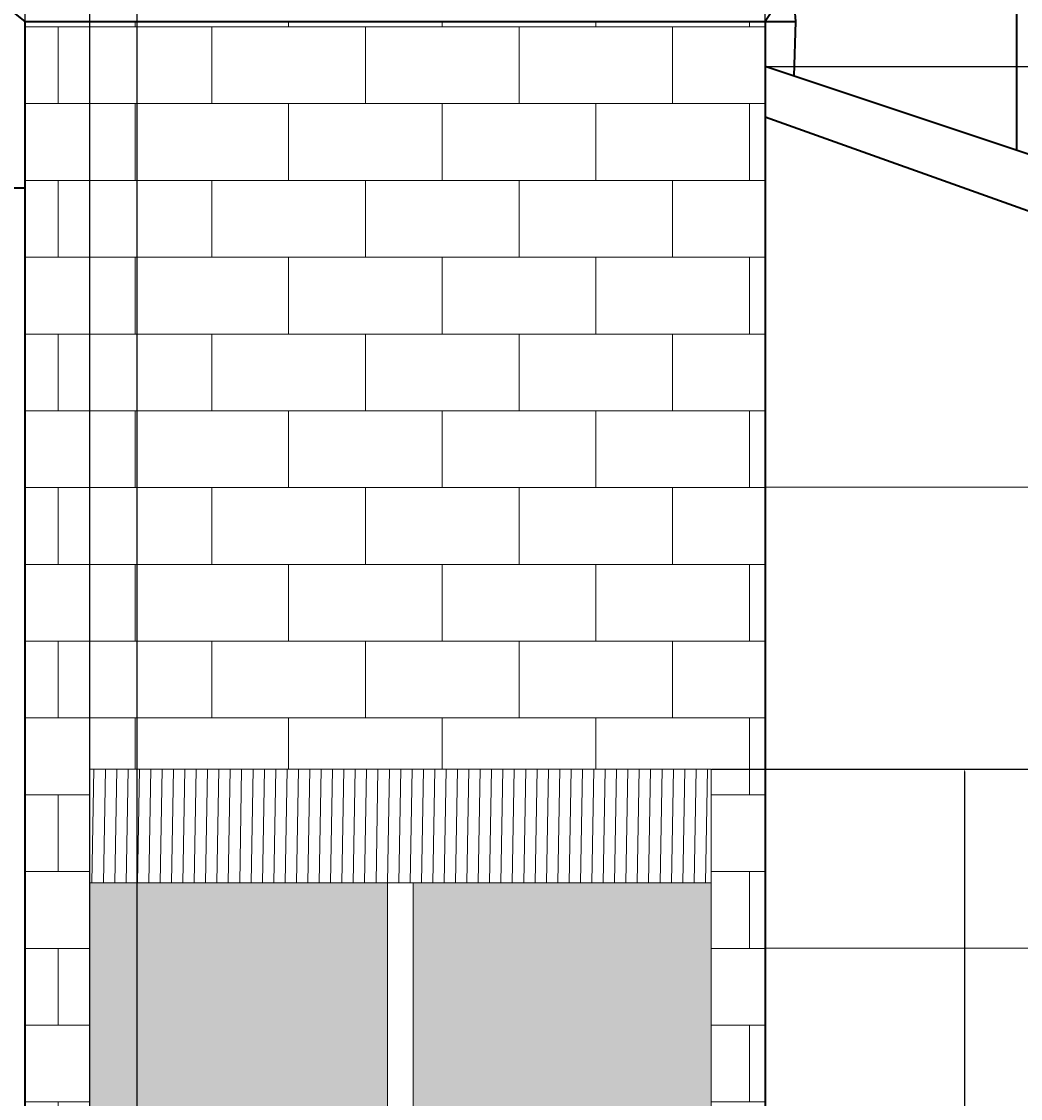
# Model space of a CAD drawing. Units: inches. Extents: x -26 to 776, y -22 to 650.
# Tile 34 of 62: x 231 to 309, y 420 to 504. Entities that reach past the tile are written whole.
import ezdxf

# ---------------------------------------------------------------- set-up
doc = ezdxf.new("R2010")
doc.units = ezdxf.units.IN
doc.header["$MEASUREMENT"] = 0
for name, color, linetype, lineweight in [('A-ANNO-DIMS', 2, 'Continuous', 18), ('A-DETL-PATT', 8, 'Continuous', 13), ('A-GLAZ', 4, 'Continuous', 18), ('A-GLAZ-PATT', 9, 'Continuous', 13), ('A-ROOF', 7, 'Continuous', 35), ('A-WALL', 7, 'Continuous', 35), ('A-WALL-PATT', 8, 'Continuous', 13)]:
    doc.layers.add(name, color=color, linetype=linetype, lineweight=lineweight)
doc.styles.get("Standard").update_dxf_attribs({"font": 'arial.ttf'})
doc.dimstyles.get("Standard").update_dxf_attribs({"dimtxt": 0.5625, "dimasz": 0.18, "dimexe": 0.18, "dimexo": 0.0625, "dimgap": 0.09, "dimtad": 0, "dimtih": 1, "dimtoh": 1, "dimdec": 4, "dimzin": 0, "dimdsep": 46, "dimlunit": 4, "dimtxsty": 'Standard', "dimcen": 0.09, "dimadec": 0, "dimazin": 0, "dimtfac": 1, "dimtdec": 4, "dimtofl": 0, "dimtmove": 0, "dimatfit": 3, "dimfxl": 1, "dimtolj": 1, "dimtzin": 0, "dimarcsym": 0})

# ---------------------------------------------------------------- blocks, each defined once
blk = doc.blocks.new('WIN-ELEV-2X4-HEAD')
for p, q in [((0, 123), (0, 131.888)), ((0, 131.888), (48.553, 131.888)), ((48.553, 131.888), (48.553, 123)), ((23.276, 0), (23.276, 123)), ((25.276, 0), (25.276, 123))]:
    blk.add_line(p, q)
blk.add_lwpolyline([(48.553, 0), (0, 0), (0, 123), (48.553, 123)], close=True)
blk = doc.blocks.new('*D9')
at = {"layer": 'A-ANNO-DIMS', "color": 0, "lineweight": -2, "transparency": 16777216}
for p, q in [((285.08, 446.006), (304.981, 446.006)), ((304.801, 445.826), (304.801, 380.444)), ((304.801, 314.299), (304.801, 379.681)), ((285.08, 314.119), (304.981, 314.119))]:
    blk.add_line(p, q, dxfattribs=at)
at = {"layer": 'A-ANNO-DIMS', "color": 0, "transparency": 16777216}
for points in [[(304.771, 445.826), (304.831, 445.826), (304.801, 446.006)], [(304.771, 314.299), (304.831, 314.299), (304.801, 314.119)]]:
    blk.add_solid(points, dxfattribs=at)
at = {"layer": 'Defpoints', "color": 0, "transparency": 16777216}
for p in [(285.018, 446.006), (304.801, 446.006), (285.018, 314.119)]:
    blk.add_point(p, dxfattribs=at)
at = {"layer": 'A-ANNO-DIMS', "color": 0, "transparency": 16777216, "insert": (304.801, 380.063), "char_height": 0.5625, "attachment_point": 5}
blk.add_mtext('\\A1;NARROW WINDOW 132 TYP.', dxfattribs=at)
blk = doc.blocks.new('*D15')
at = {"layer": 'A-ANNO-DIMS', "color": 0, "lineweight": -2, "transparency": 16777216}
for p, q in [((11.107, 491.489), (11.107, 649.856)), ((11.287, 649.676), (120.222, 649.676)), ((231.245, 649.676), (122.31, 649.676)), ((231.425, 491.489), (231.425, 649.856))]:
    blk.add_line(p, q, dxfattribs=at)
at = {"layer": 'A-ANNO-DIMS', "color": 0, "transparency": 16777216}
for points in [[(11.287, 649.706), (11.287, 649.646), (11.107, 649.676)], [(231.245, 649.706), (231.245, 649.646), (231.425, 649.676)]]:
    blk.add_solid(points, dxfattribs=at)
at = {"layer": 'Defpoints', "color": 0, "transparency": 16777216}
for p in [(231.425, 649.676), (11.107, 491.427), (231.425, 491.427)]:
    blk.add_point(p, dxfattribs=at)
at = {"layer": 'A-ANNO-DIMS', "color": 0, "transparency": 16777216, "insert": (121.266, 649.676), "char_height": 0.5625, "attachment_point": 5}
blk.add_mtext('\\A1;220.3', dxfattribs=at)
blk = doc.blocks.new('*D31')
at = {"layer": 'A-ANNO-DIMS', "color": 0, "lineweight": -2, "transparency": 16777216}
for p, q in [((289.305, 500.896), (775.335, 500.896)), ((775.155, 500.716), (775.155, 473.828)), ((775.155, 446.186), (775.155, 473.074)), ((285.08, 446.006), (775.335, 446.006))]:
    blk.add_line(p, q, dxfattribs=at)
at = {"layer": 'A-ANNO-DIMS', "color": 0, "transparency": 16777216}
for points in [[(775.125, 500.716), (775.185, 500.716), (775.155, 500.896)], [(775.125, 446.186), (775.185, 446.186), (775.155, 446.006)]]:
    blk.add_solid(points, dxfattribs=at)
at = {"layer": 'Defpoints', "color": 0, "transparency": 16777216}
for p in [(289.242, 500.896), (775.155, 500.896), (285.018, 446.006)]:
    blk.add_point(p, dxfattribs=at)
at = {"layer": 'A-ANNO-DIMS', "color": 0, "transparency": 16777216, "insert": (775.155, 473.451), "char_height": 0.5625, "attachment_point": 5}
blk.add_mtext('\\A1;54.89', dxfattribs=at)
blk = doc.blocks.new('*D34')
at = {"layer": 'A-ANNO-DIMS', "color": 0, "lineweight": -2, "transparency": 16777216}
for p, q in [((228.573, 528.296), (228.573, -21.315)), ((357.303, 528.361), (357.303, -21.315)), ((228.753, -21.135), (291.707, -21.135)), ((357.123, -21.135), (294.17, -21.135))]:
    blk.add_line(p, q, dxfattribs=at)
at = {"layer": 'A-ANNO-DIMS', "color": 0, "transparency": 16777216}
for points in [[(228.753, -21.105), (228.753, -21.165), (228.573, -21.135)], [(357.123, -21.105), (357.123, -21.165), (357.303, -21.135)]]:
    blk.add_solid(points, dxfattribs=at)
at = {"layer": 'Defpoints', "color": 0, "transparency": 16777216}
for p in [(357.303, 528.423), (228.573, 528.358), (357.303, -21.135)]:
    blk.add_point(p, dxfattribs=at)
at = {"layer": 'A-ANNO-DIMS', "color": 0, "transparency": 16777216, "insert": (292.938, -21.135), "char_height": 0.5625, "attachment_point": 5}
blk.add_mtext('\\A1;128.73', dxfattribs=at)
blk = doc.blocks.new('*D39')
at = {"layer": 'A-ANNO-DIMS', "color": 0, "lineweight": -2, "transparency": 16777216}
for p, q in [((289.242, 15.545), (289.242, 649.856)), ((289.422, 649.676), (356.478, 649.676)), ((425.563, 649.676), (358.508, 649.676)), ((425.743, 15.545), (425.743, 649.856))]:
    blk.add_line(p, q, dxfattribs=at)
at = {"layer": 'A-ANNO-DIMS', "color": 0, "transparency": 16777216}
for points in [[(289.422, 649.706), (289.422, 649.646), (289.242, 649.676)], [(425.563, 649.706), (425.563, 649.646), (425.743, 649.676)]]:
    blk.add_solid(points, dxfattribs=at)
at = {"layer": 'Defpoints', "color": 0, "transparency": 16777216}
for p in [(425.743, 649.676), (289.242, 15.482), (425.743, 15.482)]:
    blk.add_point(p, dxfattribs=at)
at = {"layer": 'A-ANNO-DIMS', "color": 0, "transparency": 16777216, "insert": (357.493, 649.676), "char_height": 0.5625, "attachment_point": 5}
blk.add_mtext('\\A1;136.5', dxfattribs=at)
blk = doc.blocks.new('*D43')
at = {"layer": 'A-ANNO-DIMS', "color": 0, "lineweight": -2, "transparency": 16777216}
for p, q in [((231.425, 159.545), (231.425, 649.856)), ((231.605, 649.676), (233.125, 649.676)), ((236.285, 649.676), (234.764, 649.676)), ((236.465, 171.48), (236.465, 649.856))]:
    blk.add_line(p, q, dxfattribs=at)
at = {"layer": 'A-ANNO-DIMS', "color": 0, "transparency": 16777216}
for points in [[(231.605, 649.706), (231.605, 649.646), (231.425, 649.676)], [(236.285, 649.706), (236.285, 649.646), (236.465, 649.676)]]:
    blk.add_solid(points, dxfattribs=at)
at = {"layer": 'Defpoints', "color": 0, "transparency": 16777216}
for p in [(236.465, 649.676), (236.465, 171.417), (231.425, 159.482)]:
    blk.add_point(p, dxfattribs=at)
at = {"layer": 'A-ANNO-DIMS', "color": 0, "transparency": 16777216, "insert": (233.945, 649.676), "char_height": 0.5625, "attachment_point": 5}
blk.add_mtext('\\A1;5.04', dxfattribs=at)
blk = doc.blocks.new('*D44')
at = {"layer": 'A-ANNO-DIMS', "color": 0, "lineweight": -2, "transparency": 16777216}
for p, q in [((231.425, 15.545), (231.425, 649.856)), ((231.605, 649.676), (234.975, 649.676)), ((239.985, 649.676), (236.615, 649.676)), ((240.165, 26.486), (240.165, 649.856))]:
    blk.add_line(p, q, dxfattribs=at)
at = {"layer": 'A-ANNO-DIMS', "color": 0, "transparency": 16777216}
for points in [[(231.605, 649.706), (231.605, 649.646), (231.425, 649.676)], [(239.985, 649.706), (239.985, 649.646), (240.165, 649.676)]]:
    blk.add_solid(points, dxfattribs=at)
at = {"layer": 'Defpoints', "color": 0, "transparency": 16777216}
for p in [(240.165, 649.676), (240.165, 26.424), (231.425, 15.482)]:
    blk.add_point(p, dxfattribs=at)
at = {"layer": 'A-ANNO-DIMS', "color": 0, "transparency": 16777216, "insert": (235.795, 649.676), "char_height": 0.5625, "attachment_point": 5}
blk.add_mtext('\\A1;8.74', dxfattribs=at)

msp = doc.modelspace()

# ---------------------------------------------------------------- hatches: boundary and pattern name
at = {"layer": 'A-DETL-PATT'}
h = msp.add_hatch(dxfattribs=at)
h.set_pattern_fill('ANSI31', color=256, scale=7.1, angle=44)
h.paths.add_polyline_path([(231.4249, 197.3298), (216.1056, 197.3298), (216.1056, 159.4824), (231.4249, 159.4824)])
h.paths.add_polyline_path([(236.4647, 197.3298), (231.4249, 197.3298), (231.4249, 159.4824), (276.1134, 159.4824), (276.1134, 171.4173), (236.4647, 171.4173)])
h.paths.add_polyline_path([(259.7413, 197.3298), (236.4647, 197.3298), (236.4647, 171.4173), (259.7413, 171.4173)], flags=17)
h.paths.add_polyline_path([(276.1134, 197.3298), (261.7413, 197.3298), (261.7413, 171.4173), (276.1134, 171.4173)], flags=17)
h.paths.add_polyline_path([(217.9529, 147.0781), (22.8891, 147.0781), (22.8891, 138.3844), (217.9529, 138.3844)])
h.paths.add_polyline_path([(285.0179, 152.3087), (285.0179, 159.4824), (231.4249, 159.4824), (240.1654, 144.8359), (280.6173, 144.8359)])
h.paths.add_polyline_path([(280.6173, 144.8359), (240.1654, 144.8359), (240.1654, 26.4239), (280.6173, 26.4239)])
h.paths.add_polyline_path([(274.6644, 134.8811), (274.6644, 34.0885), (245.7207, 34.0885), (245.7207, 134.8811)], flags=16)
h.paths.add_polyline_path([(285.0179, 303.3046), (236.4647, 303.3046), (236.4647, 294.4171), (285.0179, 294.4171)])
h.paths.add_polyline_path([(285.0179, 446.0063), (236.4647, 446.0063), (236.4647, 437.1188), (285.0179, 437.1188)])
at = {"layer": 'A-GLAZ-PATT'}
h = msp.add_hatch(dxfattribs=at)
h.set_pattern_fill('GOST_GLASS', color=256, scale=0.75)
h.set_pattern_definition([(45, (0, 0), (6.36396, 0), [3.75, -5.25]), (45, (1.591, 0), (6.36396, 0), [1.5, -7.5]), (45, (0, 1.591), (6.36396, 0), [1.5, -7.5])])
h.paths.add_polyline_path([(115.8402, 198.8773), (93.6448, 198.8773), (93.6448, 173.9734), (115.8402, 173.9734)])
h.paths.add_polyline_path([(144.1571, 198.8773), (115.8402, 198.8773), (115.8402, 173.9734), (144.1571, 173.9734)])
h.paths.add_polyline_path([(115.8402, 224.3396), (93.6448, 224.3396), (93.6448, 198.8773), (115.8402, 198.8773)])
h.paths.add_polyline_path([(144.1571, 248.4417), (115.8402, 248.4417), (115.8402, 224.3396), (144.1571, 224.3396)])
h.paths.add_polyline_path([(144.1571, 224.3396), (115.8402, 224.3396), (115.8402, 198.8773), (144.1571, 198.8773)])
h.paths.add_polyline_path([(170.5449, 224.3396), (144.1571, 224.3396), (144.1571, 198.8773), (170.5449, 198.8773)])
h.paths.add_polyline_path([(170.5449, 198.8773), (144.1571, 198.8773), (144.1571, 173.9734), (170.5449, 173.9734)])
h.paths.add_polyline_path([(194.6694, 198.8773), (170.5449, 198.8773), (170.5449, 173.9734), (194.6694, 173.9734)])
h.paths.add_polyline_path([(194.6694, 224.3396), (170.5449, 224.3396), (170.5449, 198.8773), (194.6694, 198.8773)])
h.paths.add_polyline_path([(194.6694, 248.4417), (170.5449, 248.4417), (170.5449, 224.3396), (194.6694, 224.3396)])
h.paths.add_polyline_path([(170.5449, 248.4417), (144.1571, 248.4417), (144.1571, 224.3396), (170.5449, 224.3396)])
h.paths.add_polyline_path([(144.1571, 269.3091), (115.8402, 269.3091), (115.8402, 248.4417), (144.1571, 248.4417)])
h.paths.add_polyline_path([(115.8402, 269.3091), (93.6448, 269.3091), (93.6448, 248.4417), (115.8402, 248.4417)])
h.paths.add_polyline_path([(115.8402, 248.4417), (93.6448, 248.4417), (93.6448, 224.3396), (115.8402, 224.3396)])
h.paths.add_polyline_path([(170.5449, 269.3091), (144.1571, 269.3091), (144.1571, 248.4417), (170.5449, 248.4417)])
h.paths.add_polyline_path([(194.6694, 269.3091), (170.5449, 269.3091), (170.5449, 248.4417), (194.6694, 248.4417)])
h.paths.add_polyline_path([(259.7413, 294.4171), (236.4647, 294.4171), (236.4647, 266.1888), (259.7413, 266.1888)])
h.paths.add_polyline_path([(285.0179, 294.4171), (261.7413, 294.4171), (261.7413, 266.1888), (285.0179, 266.1888)])
h.paths.add_polyline_path([(285.0179, 265.1888), (261.7413, 265.1888), (261.7413, 233.9172), (285.0179, 233.9172)])
h.paths.add_polyline_path([(259.7413, 265.1888), (236.4647, 265.1888), (236.4647, 233.9172), (259.7413, 233.9172)])
h.paths.add_polyline_path([(259.7413, 232.9172), (236.4647, 232.9172), (236.4647, 207.1741), (259.7413, 207.1741)])
h.paths.add_polyline_path([(285.0179, 232.9172), (261.7413, 232.9172), (261.7413, 207.1741), (285.0179, 207.1741)])
h.paths.add_polyline_path([(285.0179, 206.1741), (261.7413, 206.1741), (261.7413, 199.3298), (278.1134, 199.3298), (278.1134, 171.4173), (285.0179, 171.4173)])
h.paths.add_polyline_path([(259.7413, 206.1741), (236.4647, 206.1741), (236.4647, 199.3298), (259.7413, 199.3298)])
h.paths.add_polyline_path([(259.7413, 197.3298), (236.4647, 197.3298), (236.4647, 171.4173), (259.7413, 171.4173)])
h.paths.add_polyline_path([(276.1134, 197.3298), (261.7413, 197.3298), (261.7413, 171.4173), (276.1134, 171.4173)], flags=17)
h.paths.add_polyline_path([(255.8125, 548.0348), (228.5733, 548.0348), (228.5733, 528.3585), (255.8125, 528.3585)])
h.paths.add_polyline_path([(281.6181, 548.0348), (256.0792, 548.0348), (256.0792, 528.3585), (281.6181, 528.3585)])
h.paths.add_polyline_path([(308.8797, 548.0348), (281.789, 548.0348), (281.789, 528.3585), (308.8797, 528.3585)])
h.paths.add_polyline_path([(357.2724, 548.0995), (309.2457, 548.0348), (309.2457, 528.3585), (357.3034, 528.4233), (357.3034, 538.2614)])
h.paths.add_polyline_path([(259.7413, 437.1188), (236.4647, 437.1188), (236.4647, 408.8905), (259.7413, 408.8905)])
h.paths.add_polyline_path([(285.0179, 437.1188), (261.7413, 437.1188), (261.7413, 408.8905), (285.0179, 408.8905)])
h.paths.add_polyline_path([(259.7413, 407.8905), (236.4647, 407.8905), (236.4647, 376.6189), (259.7413, 376.6189)])
h.paths.add_polyline_path([(285.0179, 407.8905), (261.7413, 407.8905), (261.7413, 376.6189), (285.0179, 376.6189)])
h.paths.add_polyline_path([(285.0179, 375.6189), (261.7413, 375.6189), (261.7413, 349.8758), (285.0179, 349.8758)])
h.paths.add_polyline_path([(285.0179, 348.8758), (261.7413, 348.8758), (261.7413, 314.119), (285.0179, 314.119)])
h.paths.add_polyline_path([(259.7413, 348.8758), (236.4647, 348.8758), (236.4647, 314.119), (259.7413, 314.119)])
h.paths.add_polyline_path([(259.7413, 375.6189), (236.4647, 375.6189), (236.4647, 349.8758), (259.7413, 349.8758)])
h.paths.add_polyline_path([(194.6694, 404.1909), (170.5449, 404.1909), (170.5449, 383.3235), (194.6694, 383.3235)])
h.paths.add_polyline_path([(170.5449, 404.1909), (144.1571, 404.1909), (144.1571, 383.3235), (170.5449, 383.3235)])
h.paths.add_polyline_path([(144.1571, 404.1909), (115.8402, 404.1909), (115.8402, 383.3235), (144.1571, 383.3235)])
h.paths.add_polyline_path([(115.8402, 404.1909), (93.6448, 404.1909), (93.6448, 383.3235), (115.8402, 383.3235)])
h.paths.add_polyline_path([(115.8402, 383.3235), (93.6448, 383.3235), (93.6448, 359.2214), (115.8402, 359.2214)])
h.paths.add_polyline_path([(144.1571, 383.3235), (115.8402, 383.3235), (115.8402, 359.2214), (144.1571, 359.2214)])
h.paths.add_polyline_path([(115.8402, 359.2214), (93.6448, 359.2214), (93.6448, 333.7591), (115.8402, 333.7591)])
h.paths.add_polyline_path([(144.1571, 359.2214), (115.8402, 359.2214), (115.8402, 333.7591), (144.1571, 333.7591)])
h.paths.add_polyline_path([(115.8402, 333.7591), (93.6448, 333.7591), (93.6448, 308.8552), (115.8402, 308.8552)])
h.paths.add_polyline_path([(144.1571, 333.7591), (115.8402, 333.7591), (115.8402, 308.8552), (144.1571, 308.8552)])
h.paths.add_polyline_path([(170.5449, 333.7591), (144.1571, 333.7591), (144.1571, 308.8552), (170.5449, 308.8552)])
h.paths.add_polyline_path([(170.5449, 359.2214), (144.1571, 359.2214), (144.1571, 333.7591), (170.5449, 333.7591)])
h.paths.add_polyline_path([(170.5449, 383.3235), (144.1571, 383.3235), (144.1571, 359.2214), (170.5449, 359.2214)])
h.paths.add_polyline_path([(194.6694, 383.3235), (170.5449, 383.3235), (170.5449, 359.2214), (194.6694, 359.2214)])
h.paths.add_polyline_path([(194.6694, 359.2214), (170.5449, 359.2214), (170.5449, 333.7591), (194.6694, 333.7591)])
h.paths.add_polyline_path([(194.6694, 333.7591), (170.5449, 333.7591), (170.5449, 308.8552), (194.6694, 308.8552)])
at = {"layer": 'A-WALL-PATT'}
h = msp.add_hatch(dxfattribs=at)
h.set_pattern_fill('AR-B816', color=256, scale=0.75)
h.paths.add_polyline_path([(289.2424, 504.4205), (231.4249, 504.4205), (231.4249, 458.1203), (231.4249, 221.6413), (231.4249, 209.6413), (231.4249, 159.4824), (285.0179, 159.4824), (285.0179, 171.4173), (236.4647, 171.4173), (236.4647, 294.4171), (236.4647, 303.3046), (285.0179, 303.3046), (285.0179, 294.4171), (285.0179, 171.4173), (285.0179, 159.4824), (289.2424, 159.4824), (289.2424, 291.1798), (289.2424, 458.1203)])
h.paths.add_polyline_path([(285.0179, 446.0063), (285.0179, 437.1188), (285.0179, 314.119), (236.4647, 314.119), (236.4647, 437.1188), (236.4647, 446.0063)], flags=16)
h = msp.add_hatch(dxfattribs=at)
h.set_pattern_fill('AR-B816', color=256, scale=4.5)
h.paths.add_polyline_path([(425.7434, 448.2114), (289.2424, 496.9554), (289.2424, 458.1203), (289.2424, 291.1798), (289.2424, 20.7937), (425.7434, 20.7937), (425.7434, 283.2492)])

# ---------------------------------------------------------------- linework, layer by layer
at = {"layer": 'A-ROOF'}
for p, q in [((231.4249, 504.4205), (227.4501, 507.6108)), ((291.3688, 507.6108), (289.2424, 504.4205)), ((291.3688, 507.6108), (291.6017, 504.4205)), ((231.4249, 504.4205), (289.2424, 504.4205)), ((289.2424, 504.4205), (291.6017, 504.4205)), ((291.6017, 504.4205), (291.4864, 500.1492)), ((425.7434, 455.4717), (289.2424, 500.896)), ((425.7434, 448.2114), (289.2424, 496.9554))]:
    msp.add_line(p, q, dxfattribs=at)
at = {"layer": 'A-WALL'}
for p, q in [((308.8797, 552.4655), (308.8797, 494.3612)), ((231.4249, 458.1203), (231.4249, 504.4205)), ((289.2424, 504.4205), (289.2424, 458.1203)), ((11.1074, 491.4269), (231.4249, 491.4269)), ((231.4249, 221.6413), (231.4249, 458.1203)), ((289.2424, 458.1203), (289.2424, 291.1798))]:
    msp.add_line(p, q, dxfattribs=at)

# ---------------------------------------------------------------- block references
at = {"layer": 'A-GLAZ'}
msp.add_blockref('WIN-ELEV-2X4-HEAD', (236.465, 314.1187), dxfattribs=at)

# ---------------------------------------------------------------- dimensions: what is measured, and where the dimension line sits
at = {"layer": 'A-ANNO-DIMS'}
for base, p1, p2, override, picture, middle in [((231.4249, 649.6763), (11.1074, 491.4269), (231.4249, 491.4269), {"dimdec": 1, "dimlfac": 1, "dimrnd": 0, "dimzin": 0, "dimdsep": 46, "dimlunit": 2}, '*D15', (121.2661, 649.6763)), ((236.4647, 649.6763), (231.4249, 159.4824), (236.4647, 171.4173), {"dimdec": 2, "dimlfac": 1, "dimrnd": 0, "dimzin": 0, "dimdsep": 46, "dimlunit": 2}, '*D43', (233.9448, 649.6763)), ((240.1654, 649.6763), (231.4249, 15.4824), (240.1654, 26.4239), {"dimdec": 2, "dimlfac": 1, "dimrnd": 0, "dimzin": 0, "dimdsep": 46, "dimlunit": 2}, '*D44', (235.7952, 649.6763)), ((425.7434, 649.6763), (289.2424, 15.4824), (425.7434, 15.4824), {"dimdec": 1, "dimlfac": 1, "dimrnd": 0, "dimzin": 0, "dimdsep": 46, "dimlunit": 2}, '*D39', (357.4929, 649.6763)), ((357.3034, -21.1349), (228.5733, 528.3585), (357.3034, 528.4233), {"dimdec": 2, "dimlfac": 1, "dimrnd": 0, "dimzin": 0, "dimdsep": 46, "dimlunit": 2}, '*D34', (292.9384, -21.1349))]:
    dim = msp.add_linear_dim(base=base, p1=p1, p2=p2, dimstyle='Standard', override=override, dxfattribs=at)
    dim.commit()
    dim.dimension.update_dxf_attribs({"geometry": picture, "text_midpoint": middle})
dim = msp.add_linear_dim(base=(775.1553, 500.896), p1=(285.0179, 446.0063), p2=(289.2424, 500.896), angle=90, dimstyle='Standard', override={"dimdec": 2, "dimlfac": 1, "dimrnd": 0, "dimzin": 0, "dimdsep": 46, "dimlunit": 2}, dxfattribs=at)
dim.commit()
dim.dimension.update_dxf_attribs({"geometry": '*D31', "text_midpoint": (775.1553, 473.4511)})
dim = msp.add_linear_dim(base=(304.801, 446.0063), p1=(285.0179, 314.119), p2=(285.0179, 446.0063), angle=90, text='NARROW WINDOW <> TYP.', dimstyle='Standard', override={"dimdec": 0, "dimlfac": 1, "dimrnd": 0, "dimzin": 0, "dimdsep": 46, "dimlunit": 2}, dxfattribs=at)
dim.commit()
dim.dimension.update_dxf_attribs({"geometry": '*D9', "text_midpoint": (304.801, 380.0626)})

doc.saveas('drawing.dxf')
